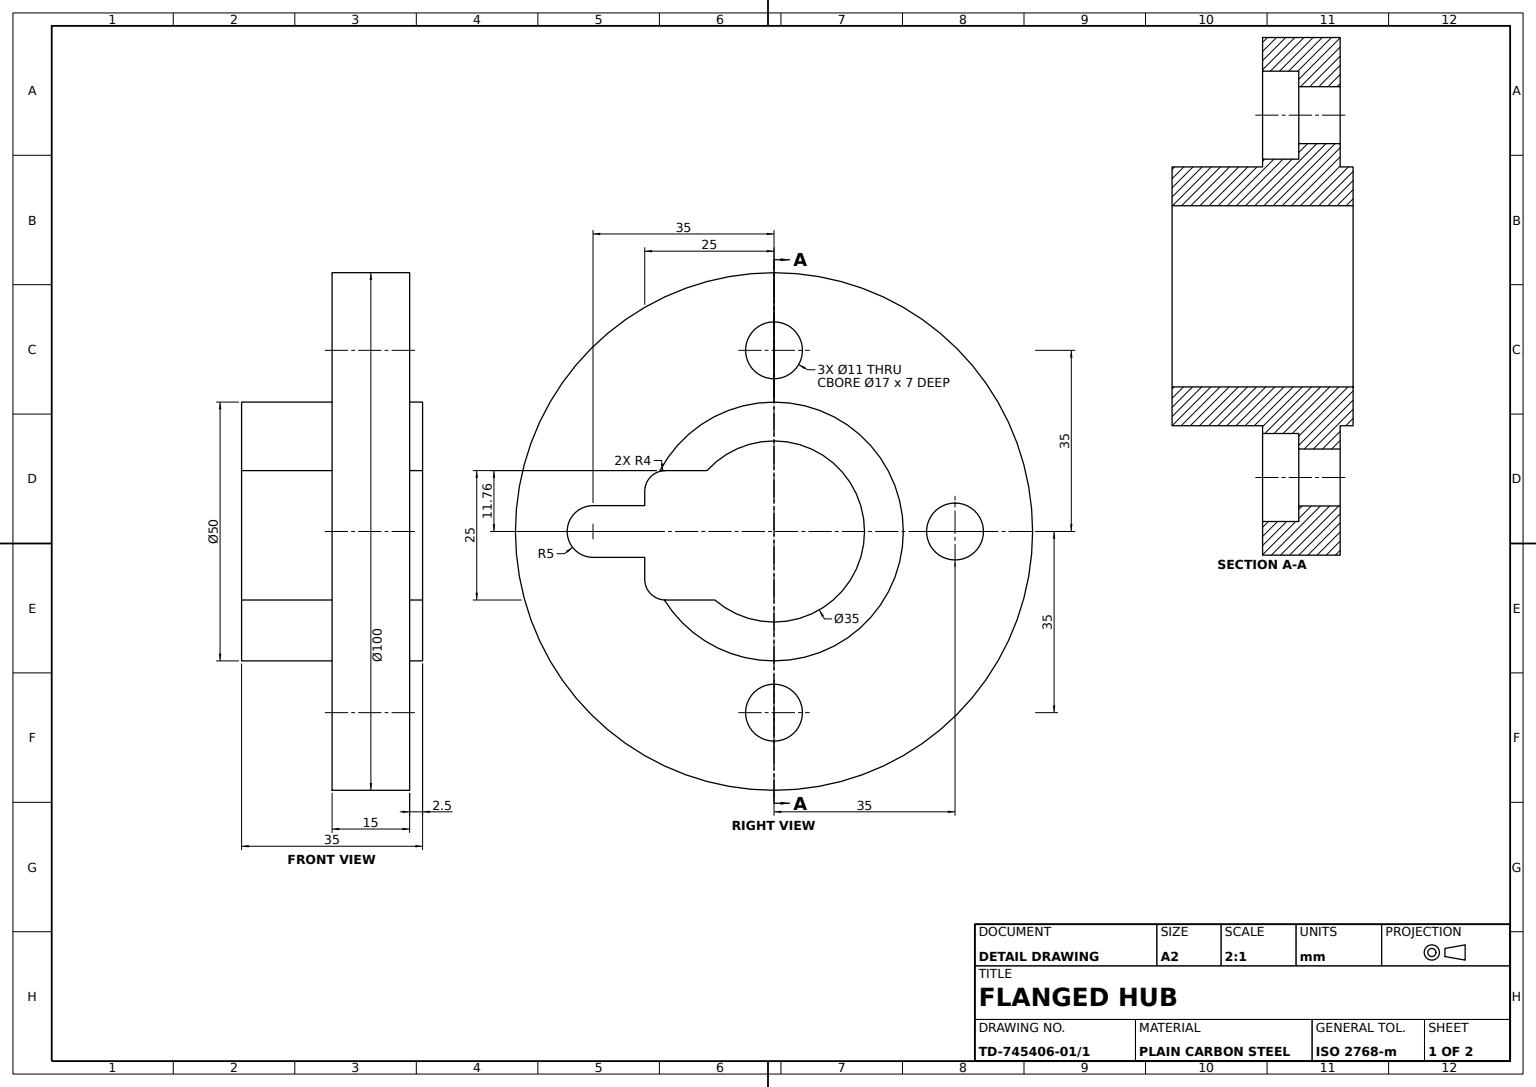
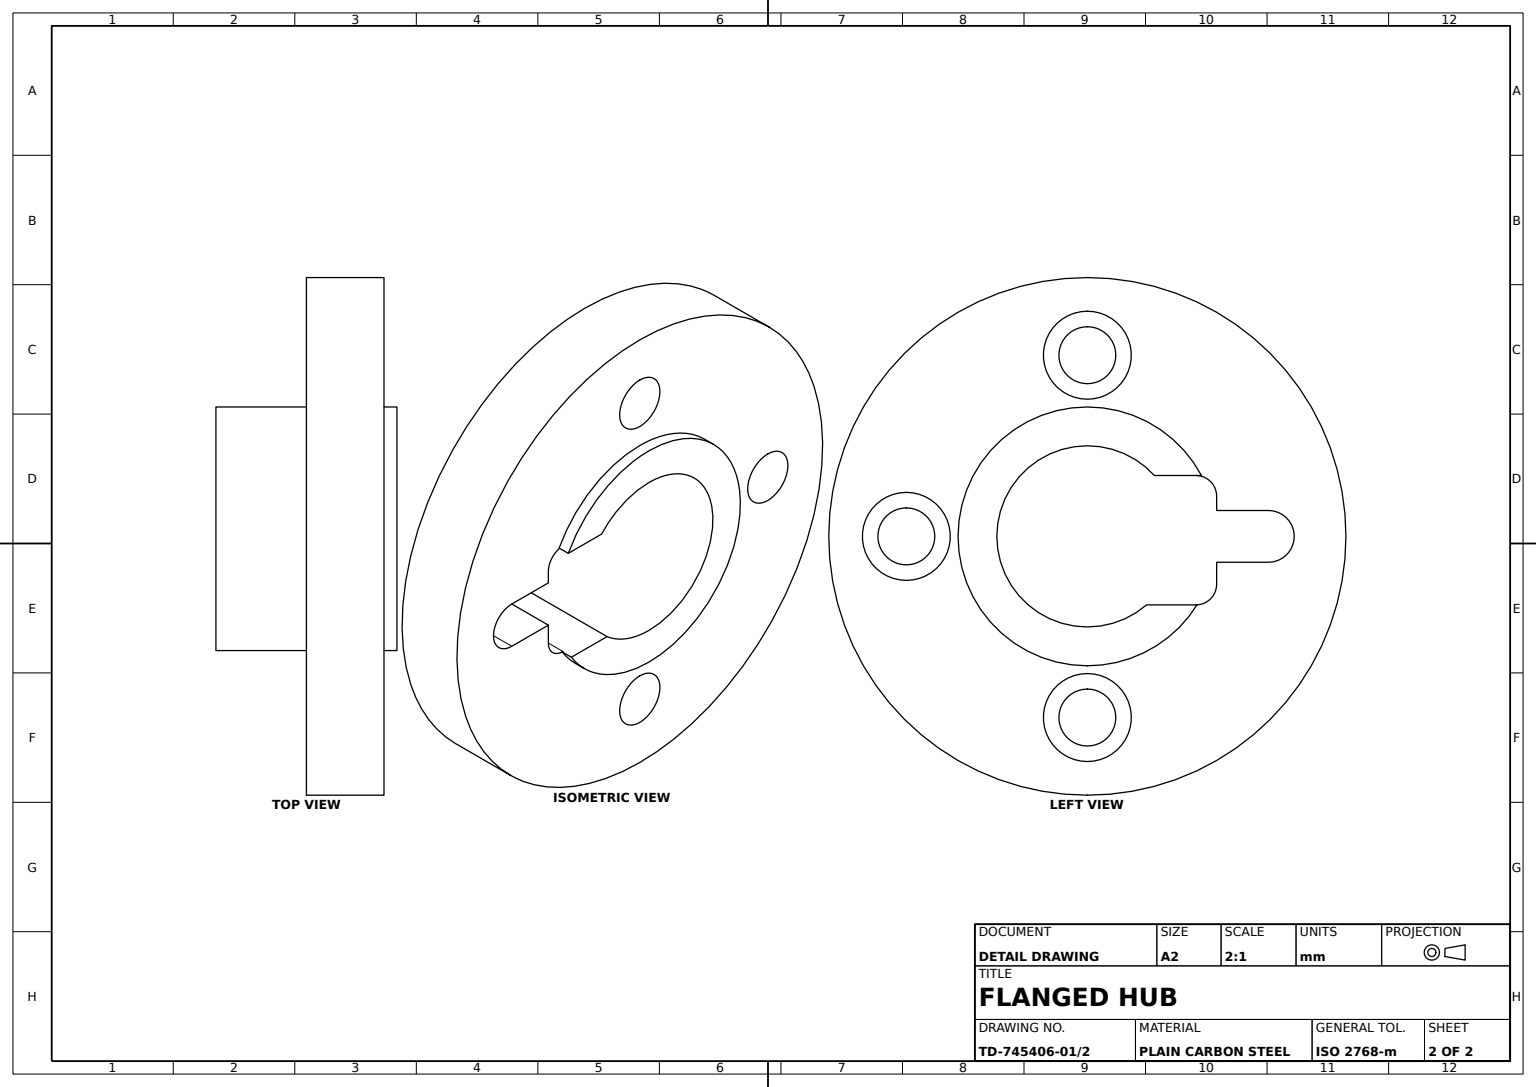
SolidWorks part; units mm, degrees
material "Plain Carbon Steel"
ref_plane "Front Plane" through (0, 0, 0) normal (0, 0, 1) x (1, 0, 0)
ref_plane "Top Plane" through (0, 0, 0) normal (0, 1, 0) x (1, 0, 0)
ref_plane "Right Plane" through (0, 0, 0) normal (1, 0, 0) x (0, 0, -1)
sketch "Flange Profile Sketch" plane through (0, 0, 0) normal (0, 0, 1) x (1, 0, 0)
  line L0 (0, 35) -> (0, 25) construction
  line L2 (-11.763, 12.9569) -> (-11.763, 21)
  line L3 (-7.763, 25) -> (-5, 25)
  line L4 (13.237, 11.4469) -> (13.237, 21)
  line L7 (5, 35) -> (5, 25)
  line L8 (-5, 35) -> (-5, 25)
  line L9 (5, 25) -> (9.237, 25)
  circle A0 centre (0, 0) radius 50
  circle A1 centre (0, 0) radius 35 construction
  arc A2 (-11.763, 12.9569) -> (13.237, 11.4469) centre (0, 0) ccw
  circle A4 centre (-35, 0) radius 5.5
  circle A5 centre (0, 35) radius 5.5 [skipped]
  circle A6 centre (35, 0) radius 5.5
  circle A7 centre (0, -35) radius 5.5
  arc A10 (5, 35) -> (-5, 35) centre (0, 35) ccw
  arc A12 (9.237, 25) -> (13.237, 21) centre (9.237, 21) cw
  arc A13 (-7.763, 25) -> (-11.763, 21) centre (-7.763, 21) ccw
  point P16 (0, 0)
  point P20 (0, 30)
  point P27 (13.237, 25)
  dimension "D1" = 100
  dimension "D2" = 70
  dimension "D3" = 35
  dimension "D4" = 11
  dimension "D8" = 5
  dimension "D9" = 4
  dimension "D6" = 11.763
  dimension "D7" = 25
  dimension "D5" = 4
extrude "Flange Ø100" add sketch "Flange Profile Sketch" along normal mid plane 15
sketch "Hub Profile Sketch" plane through (0, 0, 7.5) normal (0, 0, 1) x (1, 0, 0)
  line L0 (-11.763, 12.9569) -> (-11.763, 22.0597)
  line L1 (13.237, 11.4469) -> (13.237, 21.2081)
  line L2 (-5, 35) -> (-5, 25) construction
  arc A0 (-11.763, 12.9569) -> (13.237, 11.4469) centre (0, 0) ccw
  arc A1 (-11.763, 22.0597) -> (13.237, 21.2081) centre (0, 0) ccw
  dimension "D1" = 50
  dimension "D2" = 6.763
extrude "Hub Ø50" add sketch "Hub Profile Sketch" along normal mid plane 35
sketch "Hub Slots Sketch" plane through (0, 0, 7.5) normal (0, 0, 1) x (1, 0, 0)
  circle A0 centre (0, 0) radius 35 construction
  circle A1 centre (-35, 0) radius 8.5
  circle A2 centre (0, 35) radius 8.5 [skipped]
  circle A3 centre (35, 0) radius 8.5
  circle A4 centre (0, -35) radius 8.5
  point P15 (0, 0)
  dimension "D1" = 17
  dimension "D2" = 4
extrude "Hub Slots 4x" cut sketch "Hub Slots Sketch" against normal blind 7
